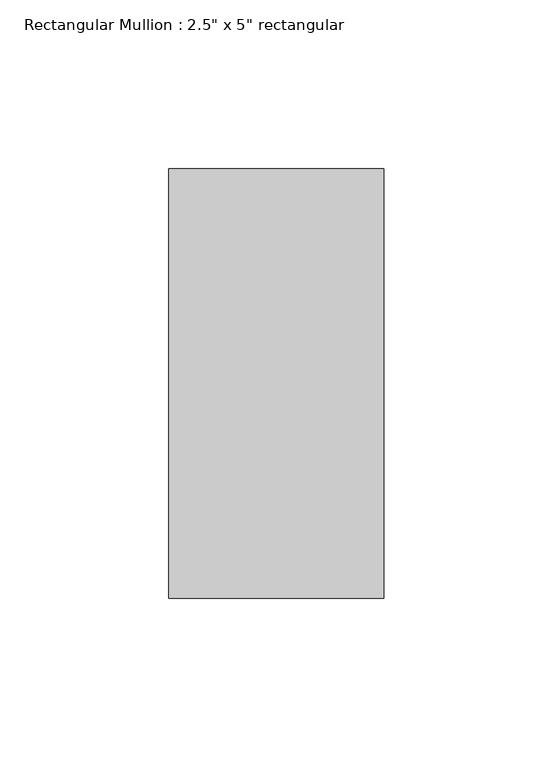
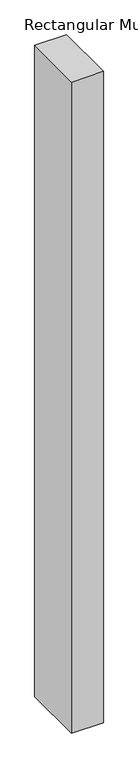
"""IFC4 building model written with IfcOpenShell, lengths in millimetres: member geometry."""

from ifc_helpers import new_model, si_unit, frame, origin, place, context, project, spatial, polyline, outline, extrude, source, transform, mapped, element, save


def member_824a4a8d(model_context):
    return source(origin(), model_context, "Body", "SweptSolid", [
        extrude(outline(polyline([(31.75, 63.5), (31.75, -63.5), (-31.75, -63.5), (-31.75, 63.5), (31.75, 63.5)])), frame((0.0, 0.0, -1371.6), z_axis=(0.0, 0.0, 1.0), x_axis=(1.0, 0.0, 0.0)), (0.0, 0.0, 1.0), 1371.6),
    ])


if __name__ == "__main__":
    model = new_model("IFC4")
    model_context = context("Model", 3, world=origin())
    ifc_project = project(units=[si_unit("LENGTHUNIT", "METRE", prefix="MILLI")], contexts=[model_context])
    site = spatial("IfcSite", under=ifc_project)
    building = spatial("IfcBuilding", under=site)
    placement = place(None, origin())
    member_shape = member_824a4a8d(model_context)
    element("IfcMember", 1, ObjectType="Rectangular Mullion : 2.5\" x 5\" rectangular", at=placement, inside=building, context=model_context, shape_type="MappedRepresentation", body=[
        mapped(member_shape, transform((0.0, 0.0, 0.0), x_axis=(1.0, 0.0, 0.0), y_axis=(0.0, 1.0, 0.0), z_axis=(0.0, 0.0, 1.0))),
    ])
    save(model, "model.ifc")

# Revit data of these elements
# Type "Rectangular Mullion : 2.5\" x 5\" rectangular"
#   built-in parameter 1007304 = 0.416667 (stored number, unit not read)
#   built-in parameter 1007301 = 0.104167 (stored number, unit not read)
#   built-in parameter 1007300 = 0.104167 (stored number, unit not read)
